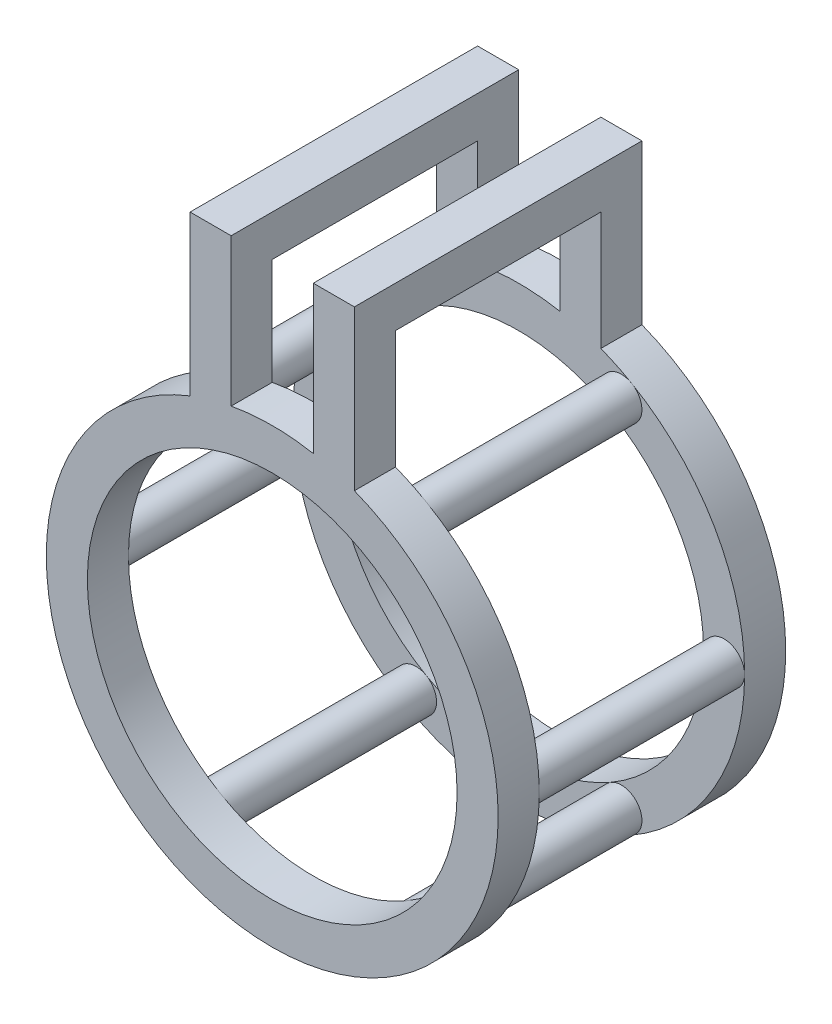
ISO-10303-21;
HEADER;
FILE_DESCRIPTION(('STEP AP214'),'2;1');
FILE_NAME('part.step','',(''),(''),'','','');
FILE_SCHEMA(('AUTOMOTIVE_DESIGN { 1 0 10303 214 1 1 1 1 }'));
ENDSEC;
DATA;
#1=APPLICATION_CONTEXT('core data for automotive mechanical design processes');
#2=APPLICATION_PROTOCOL_DEFINITION('international standard','automotive_design',2000,#1);
#3=PRODUCT_CONTEXT('',#1,'mechanical');
#4=PRODUCT('Part','Part','',(#3));
#5=PRODUCT_RELATED_PRODUCT_CATEGORY('part','',(#4));
#6=PRODUCT_DEFINITION_FORMATION('','',#4);
#7=PRODUCT_DEFINITION_CONTEXT('part definition',#1,'design');
#8=PRODUCT_DEFINITION('design','',#6,#7);
#9=PRODUCT_DEFINITION_SHAPE('','',#8);
#10=(LENGTH_UNIT() NAMED_UNIT(*) SI_UNIT(.MILLI.,.METRE.));
#11=(NAMED_UNIT(*) PLANE_ANGLE_UNIT() SI_UNIT($,.RADIAN.));
#12=(NAMED_UNIT(*) SI_UNIT($,.STERADIAN.) SOLID_ANGLE_UNIT());
#13=UNCERTAINTY_MEASURE_WITH_UNIT(LENGTH_MEASURE(1.E-05),#10,'distance_accuracy_value','');
#14=(GEOMETRIC_REPRESENTATION_CONTEXT(3) GLOBAL_UNCERTAINTY_ASSIGNED_CONTEXT((#13)) GLOBAL_UNIT_ASSIGNED_CONTEXT((#10,
#11,#12)) REPRESENTATION_CONTEXT('',''));
#15=CARTESIAN_POINT('',(0.,0.,0.));
#16=DIRECTION('',(0.,0.,1.));
#17=DIRECTION('',(1.,0.,0.));
#18=AXIS2_PLACEMENT_3D('',#15,#16,#17);
#19=CARTESIAN_POINT('',(0.,0.,-10.));
#20=DIRECTION('',(0.,0.,1.));
#21=DIRECTION('',(1.,0.,0.));
#22=AXIS2_PLACEMENT_3D('',#19,#20,#21);
#23=PLANE('',#22);
#24=CARTESIAN_POINT('',(-25.0000000000005,43.3012701892216,-10.));
#25=DIRECTION('',(0.,0.,-1.));
#26=DIRECTION('',(-1.,0.,0.));
#27=AXIS2_PLACEMENT_3D('',#24,#25,#26);
#28=CIRCLE('',#27,5.);
#29=CARTESIAN_POINT('',(-22.5000000000005,38.9711431702995,-10.));
#30=VERTEX_POINT('',#29);
#31=CARTESIAN_POINT('',(-27.5000000000006,47.6313972081438,-10.));
#32=VERTEX_POINT('',#31);
#33=EDGE_CURVE('E533',#30,#32,#28,.T.);
#34=ORIENTED_EDGE('',*,*,#33,.F.);
#35=CARTESIAN_POINT('',(0.,0.,-10.));
#36=DIRECTION('',(0.,0.,1.));
#37=DIRECTION('',(1.,0.,0.));
#38=AXIS2_PLACEMENT_3D('',#35,#36,#37);
#39=CIRCLE('',#38,45.);
#40=CARTESIAN_POINT('',(-45.,0.,-10.));
#41=VERTEX_POINT('',#40);
#42=EDGE_CURVE('E346',#30,#41,#39,.T.);
#43=ORIENTED_EDGE('',*,*,#42,.T.);
#44=CARTESIAN_POINT('',(-50.,0.,-10.));
#45=DIRECTION('',(0.,0.,-1.));
#46=DIRECTION('',(-1.,0.,0.));
#47=AXIS2_PLACEMENT_3D('',#44,#45,#46);
#48=CIRCLE('',#47,5.);
#49=CARTESIAN_POINT('',(-55.,0.,-10.));
#50=VERTEX_POINT('',#49);
#51=EDGE_CURVE('E505',#50,#41,#48,.T.);
#52=ORIENTED_EDGE('',*,*,#51,.F.);
#53=CARTESIAN_POINT('',(0.,0.,-10.));
#54=DIRECTION('',(0.,0.,1.));
#55=DIRECTION('',(1.,0.,0.));
#56=AXIS2_PLACEMENT_3D('',#53,#54,#55);
#57=CIRCLE('',#56,55.);
#58=EDGE_CURVE('E360',#32,#50,#57,.T.);
#59=ORIENTED_EDGE('',*,*,#58,.F.);
#60=EDGE_LOOP('',(#34,#43,#52,#59));
#61=FACE_BOUND('',#60,.T.);
#62=ADVANCED_FACE('F44',(#61),#23,.F.);
#63=CARTESIAN_POINT('',(10.,80.,-60.));
#64=DIRECTION('',(0.,0.,1.));
#65=DIRECTION('',(1.,0.,0.));
#66=AXIS2_PLACEMENT_3D('',#63,#64,#65);
#67=PLANE('',#66);
#68=CARTESIAN_POINT('',(0.,0.,-60.));
#69=DIRECTION('',(0.,0.,1.));
#70=DIRECTION('',(1.,0.,0.));
#71=AXIS2_PLACEMENT_3D('',#68,#69,#70);
#72=CIRCLE('',#71,45.);
#73=CARTESIAN_POINT('',(-22.5000000000005,38.9711431702995,-60.));
#74=VERTEX_POINT('',#73);
#75=CARTESIAN_POINT('',(-45.,0.,-60.));
#76=VERTEX_POINT('',#75);
#77=EDGE_CURVE('E245',#74,#76,#72,.T.);
#78=ORIENTED_EDGE('',*,*,#77,.F.);
#79=CARTESIAN_POINT('',(-25.0000000000005,43.3012701892216,-60.));
#80=DIRECTION('',(0.,0.,-1.));
#81=DIRECTION('',(-1.,0.,0.));
#82=AXIS2_PLACEMENT_3D('',#79,#80,#81);
#83=CIRCLE('',#82,5.);
#84=CARTESIAN_POINT('',(-27.5000000000006,47.6313972081438,-60.));
#85=VERTEX_POINT('',#84);
#86=EDGE_CURVE('E70',#74,#85,#83,.T.);
#87=ORIENTED_EDGE('',*,*,#86,.T.);
#88=CARTESIAN_POINT('',(0.,0.,-60.));
#89=DIRECTION('',(0.,0.,1.));
#90=DIRECTION('',(1.,0.,0.));
#91=AXIS2_PLACEMENT_3D('',#88,#89,#90);
#92=CIRCLE('',#91,55.);
#93=CARTESIAN_POINT('',(-55.,0.,-60.));
#94=VERTEX_POINT('',#93);
#95=EDGE_CURVE('E238',#85,#94,#92,.T.);
#96=ORIENTED_EDGE('',*,*,#95,.T.);
#97=CARTESIAN_POINT('',(-50.,0.,-60.));
#98=DIRECTION('',(0.,0.,-1.));
#99=DIRECTION('',(-1.,0.,0.));
#100=AXIS2_PLACEMENT_3D('',#97,#98,#99);
#101=CIRCLE('',#100,5.);
#102=EDGE_CURVE('E430',#94,#76,#101,.T.);
#103=ORIENTED_EDGE('',*,*,#102,.T.);
#104=EDGE_LOOP('',(#78,#87,#96,#103));
#105=FACE_BOUND('',#104,.T.);
#106=ADVANCED_FACE('F236',(#105),#67,.T.);
#107=EDGE_CURVE('E58',#32,#30,#28,.T.);
#108=ORIENTED_EDGE('',*,*,#107,.F.);
#109=CARTESIAN_POINT('',(-20.,51.234753829798,-10.));
#110=VERTEX_POINT('',#109);
#111=EDGE_CURVE('E358',#110,#32,#57,.T.);
#112=ORIENTED_EDGE('',*,*,#111,.F.);
#113=DIRECTION('',(0.,1.,0.));
#114=VECTOR('',#113,1.);
#115=CARTESIAN_POINT('',(-20.,51.234753829798,-10.));
#116=LINE('',#115,#114);
#117=CARTESIAN_POINT('',(-20.,80.,-10.));
#118=VERTEX_POINT('',#117);
#119=EDGE_CURVE('E421',#110,#118,#116,.T.);
#120=ORIENTED_EDGE('',*,*,#119,.T.);
#121=DIRECTION('',(-1.,0.,0.));
#122=VECTOR('',#121,1.);
#123=CARTESIAN_POINT('',(-10.,80.,-10.));
#124=LINE('',#123,#122);
#125=CARTESIAN_POINT('',(-10.,80.,-10.));
#126=VERTEX_POINT('',#125);
#127=EDGE_CURVE('E444',#126,#118,#124,.T.);
#128=ORIENTED_EDGE('',*,*,#127,.F.);
#129=DIRECTION('',(0.,1.,0.));
#130=VECTOR('',#129,1.);
#131=CARTESIAN_POINT('',(-10.,51.234753829798,-10.));
#132=LINE('',#131,#130);
#133=CARTESIAN_POINT('',(-10.,54.0832691319598,-10.));
#134=VERTEX_POINT('',#133);
#135=EDGE_CURVE('E437',#134,#126,#132,.T.);
#136=ORIENTED_EDGE('',*,*,#135,.F.);
#137=CARTESIAN_POINT('',(10.,54.0832691319598,-10.));
#138=VERTEX_POINT('',#137);
#139=EDGE_CURVE('E353',#138,#134,#57,.T.);
#140=ORIENTED_EDGE('',*,*,#139,.F.);
#141=DIRECTION('',(0.,1.,0.));
#142=VECTOR('',#141,1.);
#143=CARTESIAN_POINT('',(10.,45.,-10.));
#144=LINE('',#143,#142);
#145=CARTESIAN_POINT('',(10.,80.,-10.));
#146=VERTEX_POINT('',#145);
#147=EDGE_CURVE('E299',#138,#146,#144,.T.);
#148=ORIENTED_EDGE('',*,*,#147,.T.);
#149=DIRECTION('',(1.,0.,0.));
#150=VECTOR('',#149,1.);
#151=CARTESIAN_POINT('',(10.,80.,-10.));
#152=LINE('',#151,#150);
#153=CARTESIAN_POINT('',(20.,80.,-10.));
#154=VERTEX_POINT('',#153);
#155=EDGE_CURVE('E320',#146,#154,#152,.T.);
#156=ORIENTED_EDGE('',*,*,#155,.T.);
#157=DIRECTION('',(0.,1.,0.));
#158=VECTOR('',#157,1.);
#159=CARTESIAN_POINT('',(20.,45.,-10.));
#160=LINE('',#159,#158);
#161=CARTESIAN_POINT('',(20.,51.234753829798,-10.));
#162=VERTEX_POINT('',#161);
#163=EDGE_CURVE('E298',#162,#154,#160,.T.);
#164=ORIENTED_EDGE('',*,*,#163,.F.);
#165=CARTESIAN_POINT('',(27.4999999999996,47.6313972081444,-10.));
#166=VERTEX_POINT('',#165);
#167=EDGE_CURVE('E359',#166,#162,#57,.T.);
#168=ORIENTED_EDGE('',*,*,#167,.F.);
#169=CARTESIAN_POINT('',(24.9999999999996,43.3012701892222,-10.));
#170=DIRECTION('',(0.,0.,-1.));
#171=DIRECTION('',(-1.,0.,0.));
#172=AXIS2_PLACEMENT_3D('',#169,#170,#171);
#173=CIRCLE('',#172,4.99999999999999);
#174=CARTESIAN_POINT('',(22.4999999999996,38.9711431703,-10.));
#175=VERTEX_POINT('',#174);
#176=EDGE_CURVE('E232',#175,#166,#173,.T.);
#177=ORIENTED_EDGE('',*,*,#176,.F.);
#178=EDGE_CURVE('E1116',#175,#30,#39,.T.);
#179=ORIENTED_EDGE('',*,*,#178,.T.);
#180=EDGE_LOOP('',(#108,#112,#120,#128,#136,#140,#148,#156,#164,#168,#177,#179));
#181=FACE_BOUND('',#180,.T.);
#182=ADVANCED_FACE('F388',(#181),#23,.F.);
#183=CARTESIAN_POINT('',(-20.,51.234753829798,-60.));
#184=VERTEX_POINT('',#183);
#185=EDGE_CURVE('E247',#184,#85,#92,.T.);
#186=ORIENTED_EDGE('',*,*,#185,.T.);
#187=EDGE_CURVE('E230',#85,#74,#83,.T.);
#188=ORIENTED_EDGE('',*,*,#187,.T.);
#189=CARTESIAN_POINT('',(22.4999999999996,38.9711431703,-60.));
#190=VERTEX_POINT('',#189);
#191=EDGE_CURVE('E457',#190,#74,#72,.T.);
#192=ORIENTED_EDGE('',*,*,#191,.F.);
#193=CARTESIAN_POINT('',(24.9999999999996,43.3012701892222,-60.));
#194=DIRECTION('',(0.,0.,-1.));
#195=DIRECTION('',(-1.,0.,0.));
#196=AXIS2_PLACEMENT_3D('',#193,#194,#195);
#197=CIRCLE('',#196,4.99999999999999);
#198=CARTESIAN_POINT('',(27.4999999999996,47.6313972081444,-60.));
#199=VERTEX_POINT('',#198);
#200=EDGE_CURVE('E480',#190,#199,#197,.T.);
#201=ORIENTED_EDGE('',*,*,#200,.T.);
#202=CARTESIAN_POINT('',(20.,51.234753829798,-60.));
#203=VERTEX_POINT('',#202);
#204=EDGE_CURVE('E255',#199,#203,#92,.T.);
#205=ORIENTED_EDGE('',*,*,#204,.T.);
#206=DIRECTION('',(0.,-1.,0.));
#207=VECTOR('',#206,1.);
#208=CARTESIAN_POINT('',(20.,80.,-60.));
#209=LINE('',#208,#207);
#210=CARTESIAN_POINT('',(20.,80.,-60.));
#211=VERTEX_POINT('',#210);
#212=EDGE_CURVE('E325',#211,#203,#209,.T.);
#213=ORIENTED_EDGE('',*,*,#212,.F.);
#214=DIRECTION('',(1.,0.,0.));
#215=VECTOR('',#214,1.);
#216=CARTESIAN_POINT('',(10.,80.,-60.));
#217=LINE('',#216,#215);
#218=CARTESIAN_POINT('',(10.,80.,-60.));
#219=VERTEX_POINT('',#218);
#220=EDGE_CURVE('E340',#219,#211,#217,.T.);
#221=ORIENTED_EDGE('',*,*,#220,.F.);
#222=DIRECTION('',(0.,-1.,0.));
#223=VECTOR('',#222,1.);
#224=CARTESIAN_POINT('',(10.,80.,-60.));
#225=LINE('',#224,#223);
#226=CARTESIAN_POINT('',(10.,54.0832691319598,-60.));
#227=VERTEX_POINT('',#226);
#228=EDGE_CURVE('E308',#219,#227,#225,.T.);
#229=ORIENTED_EDGE('',*,*,#228,.T.);
#230=CARTESIAN_POINT('',(-10.,54.0832691319598,-60.));
#231=VERTEX_POINT('',#230);
#232=EDGE_CURVE('E254',#227,#231,#92,.T.);
#233=ORIENTED_EDGE('',*,*,#232,.T.);
#234=DIRECTION('',(0.,-1.,0.));
#235=VECTOR('',#234,1.);
#236=CARTESIAN_POINT('',(-10.,80.,-60.));
#237=LINE('',#236,#235);
#238=CARTESIAN_POINT('',(-10.,80.,-60.));
#239=VERTEX_POINT('',#238);
#240=EDGE_CURVE('E415',#239,#231,#237,.T.);
#241=ORIENTED_EDGE('',*,*,#240,.F.);
#242=DIRECTION('',(-1.,0.,0.));
#243=VECTOR('',#242,1.);
#244=CARTESIAN_POINT('',(-10.,80.,-60.));
#245=LINE('',#244,#243);
#246=CARTESIAN_POINT('',(-20.,80.,-60.));
#247=VERTEX_POINT('',#246);
#248=EDGE_CURVE('E442',#239,#247,#245,.T.);
#249=ORIENTED_EDGE('',*,*,#248,.T.);
#250=DIRECTION('',(0.,-1.,0.));
#251=VECTOR('',#250,1.);
#252=CARTESIAN_POINT('',(-20.,80.,-60.));
#253=LINE('',#252,#251);
#254=EDGE_CURVE('E259',#247,#184,#253,.T.);
#255=ORIENTED_EDGE('',*,*,#254,.T.);
#256=EDGE_LOOP('',(#186,#188,#192,#201,#205,#213,#221,#229,#233,#241,#249,#255));
#257=FACE_BOUND('',#256,.T.);
#258=ADVANCED_FACE('F258',(#257),#67,.T.);
#259=CARTESIAN_POINT('',(50.,3.49148133884313E-13,-10.));
#260=DIRECTION('',(0.,0.,-1.));
#261=DIRECTION('',(-1.,0.,0.));
#262=AXIS2_PLACEMENT_3D('',#259,#260,#261);
#263=CIRCLE('',#262,4.99999999999999);
#264=CARTESIAN_POINT('',(55.,3.84062947272745E-13,-10.));
#265=VERTEX_POINT('',#264);
#266=CARTESIAN_POINT('',(45.,3.14233320495882E-13,-10.));
#267=VERTEX_POINT('',#266);
#268=EDGE_CURVE('E478',#265,#267,#263,.T.);
#269=ORIENTED_EDGE('',*,*,#268,.F.);
#270=CARTESIAN_POINT('',(27.5000000000002,-47.631397208144,-10.));
#271=VERTEX_POINT('',#270);
#272=EDGE_CURVE('E538',#271,#265,#57,.T.);
#273=ORIENTED_EDGE('',*,*,#272,.F.);
#274=CARTESIAN_POINT('',(25.0000000000002,-43.3012701892218,-10.));
#275=DIRECTION('',(0.,0.,-1.));
#276=DIRECTION('',(-1.,0.,0.));
#277=AXIS2_PLACEMENT_3D('',#274,#275,#276);
#278=CIRCLE('',#277,5.);
#279=CARTESIAN_POINT('',(22.5000000000002,-38.9711431702996,-10.));
#280=VERTEX_POINT('',#279);
#281=EDGE_CURVE('E489',#280,#271,#278,.T.);
#282=ORIENTED_EDGE('',*,*,#281,.F.);
#283=EDGE_CURVE('E1120',#280,#267,#39,.T.);
#284=ORIENTED_EDGE('',*,*,#283,.T.);
#285=EDGE_LOOP('',(#269,#273,#282,#284));
#286=FACE_BOUND('',#285,.T.);
#287=ADVANCED_FACE('F547',(#286),#23,.F.);
#288=CARTESIAN_POINT('',(27.5000000000002,-47.631397208144,-60.));
#289=VERTEX_POINT('',#288);
#290=CARTESIAN_POINT('',(55.,3.84062947272745E-13,-60.));
#291=VERTEX_POINT('',#290);
#292=EDGE_CURVE('E269',#289,#291,#92,.T.);
#293=ORIENTED_EDGE('',*,*,#292,.T.);
#294=CARTESIAN_POINT('',(50.,3.49148133884313E-13,-60.));
#295=DIRECTION('',(0.,0.,-1.));
#296=DIRECTION('',(-1.,0.,0.));
#297=AXIS2_PLACEMENT_3D('',#294,#295,#296);
#298=CIRCLE('',#297,4.99999999999999);
#299=CARTESIAN_POINT('',(45.,3.14233320495882E-13,-60.));
#300=VERTEX_POINT('',#299);
#301=EDGE_CURVE('E466',#291,#300,#298,.T.);
#302=ORIENTED_EDGE('',*,*,#301,.T.);
#303=CARTESIAN_POINT('',(22.5000000000002,-38.9711431702996,-60.));
#304=VERTEX_POINT('',#303);
#305=EDGE_CURVE('E454',#304,#300,#72,.T.);
#306=ORIENTED_EDGE('',*,*,#305,.F.);
#307=CARTESIAN_POINT('',(25.0000000000002,-43.3012701892218,-60.));
#308=DIRECTION('',(0.,0.,-1.));
#309=DIRECTION('',(-1.,0.,0.));
#310=AXIS2_PLACEMENT_3D('',#307,#308,#309);
#311=CIRCLE('',#310,5.);
#312=EDGE_CURVE('E470',#304,#289,#311,.T.);
#313=ORIENTED_EDGE('',*,*,#312,.T.);
#314=EDGE_LOOP('',(#293,#302,#306,#313));
#315=FACE_BOUND('',#314,.T.);
#316=ADVANCED_FACE('F468',(#315),#67,.T.);
#317=EDGE_CURVE('E482',#271,#280,#278,.T.);
#318=ORIENTED_EDGE('',*,*,#317,.F.);
#319=CARTESIAN_POINT('',(-27.4999999999999,-47.6313972081442,-10.));
#320=VERTEX_POINT('',#319);
#321=EDGE_CURVE('E536',#320,#271,#57,.T.);
#322=ORIENTED_EDGE('',*,*,#321,.F.);
#323=CARTESIAN_POINT('',(-24.9999999999999,-43.301270189222,-10.));
#324=DIRECTION('',(0.,0.,-1.));
#325=DIRECTION('',(-1.,0.,0.));
#326=AXIS2_PLACEMENT_3D('',#323,#324,#325);
#327=CIRCLE('',#326,5.);
#328=CARTESIAN_POINT('',(-22.4999999999999,-38.9711431702998,-10.));
#329=VERTEX_POINT('',#328);
#330=EDGE_CURVE('E500',#329,#320,#327,.T.);
#331=ORIENTED_EDGE('',*,*,#330,.F.);
#332=EDGE_CURVE('E352',#329,#280,#39,.T.);
#333=ORIENTED_EDGE('',*,*,#332,.T.);
#334=EDGE_LOOP('',(#318,#322,#331,#333));
#335=FACE_BOUND('',#334,.T.);
#336=ADVANCED_FACE('F551',(#335),#23,.F.);
#337=CARTESIAN_POINT('',(-27.4999999999999,-47.6313972081442,-60.));
#338=VERTEX_POINT('',#337);
#339=EDGE_CURVE('E264',#338,#289,#92,.T.);
#340=ORIENTED_EDGE('',*,*,#339,.T.);
#341=EDGE_CURVE('E487',#289,#304,#311,.T.);
#342=ORIENTED_EDGE('',*,*,#341,.T.);
#343=CARTESIAN_POINT('',(-22.4999999999999,-38.9711431702998,-60.));
#344=VERTEX_POINT('',#343);
#345=EDGE_CURVE('E453',#344,#304,#72,.T.);
#346=ORIENTED_EDGE('',*,*,#345,.F.);
#347=CARTESIAN_POINT('',(-24.9999999999999,-43.301270189222,-60.));
#348=DIRECTION('',(0.,0.,-1.));
#349=DIRECTION('',(-1.,0.,0.));
#350=AXIS2_PLACEMENT_3D('',#347,#348,#349);
#351=CIRCLE('',#350,5.);
#352=EDGE_CURVE('E492',#344,#338,#351,.T.);
#353=ORIENTED_EDGE('',*,*,#352,.T.);
#354=EDGE_LOOP('',(#340,#342,#346,#353));
#355=FACE_BOUND('',#354,.T.);
#356=ADVANCED_FACE('F591',(#355),#67,.T.);
#357=EDGE_CURVE('E488',#320,#329,#327,.T.);
#358=ORIENTED_EDGE('',*,*,#357,.F.);
#359=EDGE_CURVE('E530',#50,#320,#57,.T.);
#360=ORIENTED_EDGE('',*,*,#359,.F.);
#361=EDGE_CURVE('E494',#41,#50,#48,.T.);
#362=ORIENTED_EDGE('',*,*,#361,.F.);
#363=EDGE_CURVE('E349',#41,#329,#39,.T.);
#364=ORIENTED_EDGE('',*,*,#363,.T.);
#365=EDGE_LOOP('',(#358,#360,#362,#364));
#366=FACE_BOUND('',#365,.T.);
#367=ADVANCED_FACE('F581',(#366),#23,.F.);
#368=EDGE_CURVE('E252',#94,#338,#92,.T.);
#369=ORIENTED_EDGE('',*,*,#368,.T.);
#370=EDGE_CURVE('E497',#338,#344,#351,.T.);
#371=ORIENTED_EDGE('',*,*,#370,.T.);
#372=EDGE_CURVE('E296',#76,#344,#72,.T.);
#373=ORIENTED_EDGE('',*,*,#372,.F.);
#374=EDGE_CURVE('E501',#76,#94,#101,.T.);
#375=ORIENTED_EDGE('',*,*,#374,.T.);
#376=EDGE_LOOP('',(#369,#371,#373,#375));
#377=FACE_BOUND('',#376,.T.);
#378=ADVANCED_FACE('F587',(#377),#67,.T.);
#379=CARTESIAN_POINT('',(0.,0.,-10.));
#380=DIRECTION('',(0.,0.,1.));
#381=DIRECTION('',(1.,0.,0.));
#382=AXIS2_PLACEMENT_3D('',#379,#380,#381);
#383=CYLINDRICAL_SURFACE('',#382,55.);
#384=ORIENTED_EDGE('',*,*,#139,.T.);
#385=DIRECTION('',(0.,0.,1.));
#386=VECTOR('',#385,1.);
#387=CARTESIAN_POINT('',(-10.,54.0832691319598,-10.));
#388=LINE('',#387,#386);
#389=CARTESIAN_POINT('',(-10.,54.0832691319598,0.));
#390=VERTEX_POINT('',#389);
#391=EDGE_CURVE('E446',#134,#390,#388,.T.);
#392=ORIENTED_EDGE('',*,*,#391,.T.);
#393=CARTESIAN_POINT('',(0.,0.,0.));
#394=DIRECTION('',(0.,0.,1.));
#395=DIRECTION('',(1.,0.,0.));
#396=AXIS2_PLACEMENT_3D('',#393,#394,#395);
#397=CIRCLE('',#396,55.);
#398=CARTESIAN_POINT('',(10.,54.0832691319598,0.));
#399=VERTEX_POINT('',#398);
#400=EDGE_CURVE('E356',#399,#390,#397,.T.);
#401=ORIENTED_EDGE('',*,*,#400,.F.);
#402=DIRECTION('',(0.,0.,1.));
#403=VECTOR('',#402,1.);
#404=CARTESIAN_POINT('',(10.,54.0832691319598,-10.));
#405=LINE('',#404,#403);
#406=EDGE_CURVE('E341',#399,#138,#405,.F.);
#407=ORIENTED_EDGE('',*,*,#406,.T.);
#408=EDGE_LOOP('',(#384,#392,#401,#407));
#409=FACE_BOUND('',#408,.T.);
#410=ADVANCED_FACE('F524',(#409),#383,.T.);
#411=CARTESIAN_POINT('',(0.,0.,-60.));
#412=DIRECTION('',(0.,0.,-1.));
#413=DIRECTION('',(-1.,0.,0.));
#414=AXIS2_PLACEMENT_3D('',#411,#412,#413);
#415=CYLINDRICAL_SURFACE('',#414,55.);
#416=DIRECTION('',(0.,0.,-1.));
#417=VECTOR('',#416,1.);
#418=CARTESIAN_POINT('',(-10.,54.0832691319598,-60.));
#419=LINE('',#418,#417);
#420=CARTESIAN_POINT('',(-10.,54.0832691319598,-70.));
#421=VERTEX_POINT('',#420);
#422=EDGE_CURVE('E11',#231,#421,#419,.T.);
#423=ORIENTED_EDGE('',*,*,#422,.F.);
#424=ORIENTED_EDGE('',*,*,#232,.F.);
#425=DIRECTION('',(0.,0.,-1.));
#426=VECTOR('',#425,1.);
#427=CARTESIAN_POINT('',(10.,54.0832691319598,-60.));
#428=LINE('',#427,#426);
#429=CARTESIAN_POINT('',(10.,54.0832691319599,-70.));
#430=VERTEX_POINT('',#429);
#431=EDGE_CURVE('E265',#227,#430,#428,.T.);
#432=ORIENTED_EDGE('',*,*,#431,.T.);
#433=CARTESIAN_POINT('',(0.,0.,-70.));
#434=DIRECTION('',(0.,0.,1.));
#435=DIRECTION('',(1.,0.,0.));
#436=AXIS2_PLACEMENT_3D('',#433,#434,#435);
#437=CIRCLE('',#436,55.);
#438=EDGE_CURVE('E284',#430,#421,#437,.T.);
#439=ORIENTED_EDGE('',*,*,#438,.T.);
#440=EDGE_LOOP('',(#423,#424,#432,#439));
#441=FACE_BOUND('',#440,.T.);
#442=ADVANCED_FACE('F401',(#441),#415,.T.);
#443=CARTESIAN_POINT('',(10.,0.,0.));
#444=DIRECTION('',(1.,0.,0.));
#445=DIRECTION('',(0.,0.,-1.));
#446=AXIS2_PLACEMENT_3D('',#443,#444,#445);
#447=PLANE('',#446);
#448=ORIENTED_EDGE('',*,*,#431,.F.);
#449=ORIENTED_EDGE('',*,*,#228,.F.);
#450=DIRECTION('',(0.,0.,-1.));
#451=VECTOR('',#450,1.);
#452=CARTESIAN_POINT('',(10.,80.,-10.));
#453=LINE('',#452,#451);
#454=EDGE_CURVE('E305',#146,#219,#453,.T.);
#455=ORIENTED_EDGE('',*,*,#454,.F.);
#456=ORIENTED_EDGE('',*,*,#147,.F.);
#457=ORIENTED_EDGE('',*,*,#406,.F.);
#458=DIRECTION('',(0.,-1.,0.));
#459=VECTOR('',#458,1.);
#460=CARTESIAN_POINT('',(10.,45.,0.));
#461=LINE('',#460,#459);
#462=CARTESIAN_POINT('',(10.,90.,0.));
#463=VERTEX_POINT('',#462);
#464=EDGE_CURVE('E314',#463,#399,#461,.T.);
#465=ORIENTED_EDGE('',*,*,#464,.F.);
#466=DIRECTION('',(0.,0.,1.));
#467=VECTOR('',#466,1.);
#468=CARTESIAN_POINT('',(10.,90.,0.));
#469=LINE('',#468,#467);
#470=CARTESIAN_POINT('',(10.,90.,-70.));
#471=VERTEX_POINT('',#470);
#472=EDGE_CURVE('E313',#471,#463,#469,.T.);
#473=ORIENTED_EDGE('',*,*,#472,.F.);
#474=DIRECTION('',(0.,1.,0.));
#475=VECTOR('',#474,1.);
#476=CARTESIAN_POINT('',(10.,90.,-70.));
#477=LINE('',#476,#475);
#478=EDGE_CURVE('E310',#430,#471,#477,.T.);
#479=ORIENTED_EDGE('',*,*,#478,.F.);
#480=EDGE_LOOP('',(#448,#449,#455,#456,#457,#465,#473,#479));
#481=FACE_BOUND('',#480,.T.);
#482=ADVANCED_FACE('F405',(#481),#447,.F.);
#483=CARTESIAN_POINT('',(20.,0.,0.));
#484=DIRECTION('',(1.,0.,0.));
#485=DIRECTION('',(0.,0.,-1.));
#486=AXIS2_PLACEMENT_3D('',#483,#484,#485);
#487=PLANE('',#486);
#488=ORIENTED_EDGE('',*,*,#212,.T.);
#489=DIRECTION('',(0.,0.,-1.));
#490=VECTOR('',#489,1.);
#491=CARTESIAN_POINT('',(20.,51.234753829798,-60.));
#492=LINE('',#491,#490);
#493=CARTESIAN_POINT('',(20.,51.234753829798,-70.));
#494=VERTEX_POINT('',#493);
#495=EDGE_CURVE('E52',#203,#494,#492,.T.);
#496=ORIENTED_EDGE('',*,*,#495,.T.);
#497=DIRECTION('',(0.,1.,0.));
#498=VECTOR('',#497,1.);
#499=CARTESIAN_POINT('',(20.,90.,-70.));
#500=LINE('',#499,#498);
#501=CARTESIAN_POINT('',(20.,90.,-70.));
#502=VERTEX_POINT('',#501);
#503=EDGE_CURVE('E322',#494,#502,#500,.T.);
#504=ORIENTED_EDGE('',*,*,#503,.T.);
#505=DIRECTION('',(0.,0.,1.));
#506=VECTOR('',#505,1.);
#507=CARTESIAN_POINT('',(20.,90.,0.));
#508=LINE('',#507,#506);
#509=CARTESIAN_POINT('',(20.,90.,0.));
#510=VERTEX_POINT('',#509);
#511=EDGE_CURVE('E326',#502,#510,#508,.T.);
#512=ORIENTED_EDGE('',*,*,#511,.T.);
#513=DIRECTION('',(0.,-1.,0.));
#514=VECTOR('',#513,1.);
#515=CARTESIAN_POINT('',(20.,45.,0.));
#516=LINE('',#515,#514);
#517=CARTESIAN_POINT('',(20.,51.234753829798,0.));
#518=VERTEX_POINT('',#517);
#519=EDGE_CURVE('E301',#510,#518,#516,.T.);
#520=ORIENTED_EDGE('',*,*,#519,.T.);
#521=DIRECTION('',(0.,0.,1.));
#522=VECTOR('',#521,1.);
#523=CARTESIAN_POINT('',(20.,51.234753829798,-10.));
#524=LINE('',#523,#522);
#525=EDGE_CURVE('E334',#518,#162,#524,.F.);
#526=ORIENTED_EDGE('',*,*,#525,.T.);
#527=ORIENTED_EDGE('',*,*,#163,.T.);
#528=DIRECTION('',(0.,0.,-1.));
#529=VECTOR('',#528,1.);
#530=CARTESIAN_POINT('',(20.,80.,-10.));
#531=LINE('',#530,#529);
#532=EDGE_CURVE('E317',#154,#211,#531,.T.);
#533=ORIENTED_EDGE('',*,*,#532,.T.);
#534=EDGE_LOOP('',(#488,#496,#504,#512,#520,#526,#527,#533));
#535=FACE_BOUND('',#534,.T.);
#536=ADVANCED_FACE('F365',(#535),#487,.T.);
#537=DIRECTION('',(0.,0.,-1.));
#538=VECTOR('',#537,1.);
#539=CARTESIAN_POINT('',(-20.,51.234753829798,0.));
#540=LINE('',#539,#538);
#541=CARTESIAN_POINT('',(-20.,51.234753829798,0.));
#542=VERTEX_POINT('',#541);
#543=EDGE_CURVE('E436',#542,#110,#540,.T.);
#544=ORIENTED_EDGE('',*,*,#543,.T.);
#545=ORIENTED_EDGE('',*,*,#111,.T.);
#546=ORIENTED_EDGE('',*,*,#58,.T.);
#547=ORIENTED_EDGE('',*,*,#359,.T.);
#548=ORIENTED_EDGE('',*,*,#321,.T.);
#549=ORIENTED_EDGE('',*,*,#272,.T.);
#550=EDGE_CURVE('E540',#265,#166,#57,.T.);
#551=ORIENTED_EDGE('',*,*,#550,.T.);
#552=ORIENTED_EDGE('',*,*,#167,.T.);
#553=ORIENTED_EDGE('',*,*,#525,.F.);
#554=EDGE_CURVE('E355',#542,#518,#397,.T.);
#555=ORIENTED_EDGE('',*,*,#554,.F.);
#556=EDGE_LOOP('',(#544,#545,#546,#547,#548,#549,#551,#552,#553,#555));
#557=FACE_BOUND('',#556,.T.);
#558=ADVANCED_FACE('F50',(#557),#383,.T.);
#559=EDGE_CURVE('E479',#166,#175,#173,.T.);
#560=ORIENTED_EDGE('',*,*,#559,.F.);
#561=ORIENTED_EDGE('',*,*,#550,.F.);
#562=EDGE_CURVE('E473',#267,#265,#263,.T.);
#563=ORIENTED_EDGE('',*,*,#562,.F.);
#564=EDGE_CURVE('E1117',#267,#175,#39,.T.);
#565=ORIENTED_EDGE('',*,*,#564,.T.);
#566=EDGE_LOOP('',(#560,#561,#563,#565));
#567=FACE_BOUND('',#566,.T.);
#568=ADVANCED_FACE('F573',(#567),#23,.F.);
#569=CARTESIAN_POINT('',(0.,0.,0.));
#570=DIRECTION('',(0.,0.,1.));
#571=DIRECTION('',(1.,0.,0.));
#572=AXIS2_PLACEMENT_3D('',#569,#570,#571);
#573=PLANE('',#572);
#574=ORIENTED_EDGE('',*,*,#400,.T.);
#575=DIRECTION('',(0.,-1.,0.));
#576=VECTOR('',#575,1.);
#577=CARTESIAN_POINT('',(-10.,90.,0.));
#578=LINE('',#577,#576);
#579=CARTESIAN_POINT('',(-10.,90.,0.));
#580=VERTEX_POINT('',#579);
#581=EDGE_CURVE('E412',#580,#390,#578,.T.);
#582=ORIENTED_EDGE('',*,*,#581,.F.);
#583=DIRECTION('',(-1.,0.,0.));
#584=VECTOR('',#583,1.);
#585=CARTESIAN_POINT('',(-10.,90.,0.));
#586=LINE('',#585,#584);
#587=CARTESIAN_POINT('',(-20.,90.,0.));
#588=VERTEX_POINT('',#587);
#589=EDGE_CURVE('E425',#580,#588,#586,.T.);
#590=ORIENTED_EDGE('',*,*,#589,.T.);
#591=DIRECTION('',(0.,-1.,0.));
#592=VECTOR('',#591,1.);
#593=CARTESIAN_POINT('',(-20.,90.,0.));
#594=LINE('',#593,#592);
#595=EDGE_CURVE('E383',#588,#542,#594,.T.);
#596=ORIENTED_EDGE('',*,*,#595,.T.);
#597=ORIENTED_EDGE('',*,*,#554,.T.);
#598=ORIENTED_EDGE('',*,*,#519,.F.);
#599=DIRECTION('',(1.,0.,0.));
#600=VECTOR('',#599,1.);
#601=CARTESIAN_POINT('',(10.,90.,0.));
#602=LINE('',#601,#600);
#603=EDGE_CURVE('E332',#463,#510,#602,.T.);
#604=ORIENTED_EDGE('',*,*,#603,.F.);
#605=ORIENTED_EDGE('',*,*,#464,.T.);
#606=EDGE_LOOP('',(#574,#582,#590,#596,#597,#598,#604,#605));
#607=FACE_BOUND('',#606,.T.);
#608=CARTESIAN_POINT('',(0.,0.,0.));
#609=DIRECTION('',(0.,0.,1.));
#610=DIRECTION('',(1.,0.,0.));
#611=AXIS2_PLACEMENT_3D('',#608,#609,#610);
#612=CIRCLE('',#611,45.);
#613=CARTESIAN_POINT('',(45.,0.,0.));
#614=VERTEX_POINT('',#613);
#615=EDGE_CURVE('E344',#614,#614,#612,.T.);
#616=ORIENTED_EDGE('',*,*,#615,.F.);
#617=EDGE_LOOP('',(#616));
#618=FACE_BOUND('',#617,.T.);
#619=ADVANCED_FACE('F378',(#607,#618),#573,.T.);
#620=CARTESIAN_POINT('',(0.,0.,-70.));
#621=DIRECTION('',(0.,0.,1.));
#622=DIRECTION('',(1.,0.,0.));
#623=AXIS2_PLACEMENT_3D('',#620,#621,#622);
#624=CYLINDRICAL_SURFACE('',#623,45.);
#625=ORIENTED_EDGE('',*,*,#615,.T.);
#626=EDGE_LOOP('',(#625));
#627=FACE_BOUND('',#626,.T.);
#628=ORIENTED_EDGE('',*,*,#363,.F.);
#629=ORIENTED_EDGE('',*,*,#42,.F.);
#630=ORIENTED_EDGE('',*,*,#178,.F.);
#631=ORIENTED_EDGE('',*,*,#564,.F.);
#632=ORIENTED_EDGE('',*,*,#283,.F.);
#633=ORIENTED_EDGE('',*,*,#332,.F.);
#634=EDGE_LOOP('',(#628,#629,#630,#631,#632,#633));
#635=FACE_BOUND('',#634,.T.);
#636=ADVANCED_FACE('F586',(#627,#635),#624,.F.);
#637=CARTESIAN_POINT('',(10.,90.,0.));
#638=DIRECTION('',(0.,1.,0.));
#639=DIRECTION('',(0.,0.,1.));
#640=AXIS2_PLACEMENT_3D('',#637,#638,#639);
#641=PLANE('',#640);
#642=ORIENTED_EDGE('',*,*,#511,.F.);
#643=DIRECTION('',(1.,0.,0.));
#644=VECTOR('',#643,1.);
#645=CARTESIAN_POINT('',(10.,90.,-70.));
#646=LINE('',#645,#644);
#647=EDGE_CURVE('E331',#471,#502,#646,.T.);
#648=ORIENTED_EDGE('',*,*,#647,.F.);
#649=ORIENTED_EDGE('',*,*,#472,.T.);
#650=ORIENTED_EDGE('',*,*,#603,.T.);
#651=EDGE_LOOP('',(#642,#648,#649,#650));
#652=FACE_BOUND('',#651,.T.);
#653=ADVANCED_FACE('F374',(#652),#641,.T.);
#654=CARTESIAN_POINT('',(10.,90.,-70.));
#655=DIRECTION('',(0.,0.,-1.));
#656=DIRECTION('',(-1.,0.,0.));
#657=AXIS2_PLACEMENT_3D('',#654,#655,#656);
#658=PLANE('',#657);
#659=CARTESIAN_POINT('',(-20.,51.234753829798,-70.));
#660=VERTEX_POINT('',#659);
#661=EDGE_CURVE('E292',#660,#494,#437,.T.);
#662=ORIENTED_EDGE('',*,*,#661,.F.);
#663=DIRECTION('',(0.,1.,0.));
#664=VECTOR('',#663,1.);
#665=CARTESIAN_POINT('',(-20.,51.234753829798,-70.));
#666=LINE('',#665,#664);
#667=CARTESIAN_POINT('',(-20.,90.,-70.));
#668=VERTEX_POINT('',#667);
#669=EDGE_CURVE('E431',#660,#668,#666,.T.);
#670=ORIENTED_EDGE('',*,*,#669,.T.);
#671=DIRECTION('',(-1.,0.,0.));
#672=VECTOR('',#671,1.);
#673=CARTESIAN_POINT('',(-10.,90.,-70.));
#674=LINE('',#673,#672);
#675=CARTESIAN_POINT('',(-10.,90.,-70.));
#676=VERTEX_POINT('',#675);
#677=EDGE_CURVE('E407',#676,#668,#674,.T.);
#678=ORIENTED_EDGE('',*,*,#677,.F.);
#679=DIRECTION('',(0.,1.,0.));
#680=VECTOR('',#679,1.);
#681=CARTESIAN_POINT('',(-10.,51.234753829798,-70.));
#682=LINE('',#681,#680);
#683=EDGE_CURVE('E406',#421,#676,#682,.T.);
#684=ORIENTED_EDGE('',*,*,#683,.F.);
#685=ORIENTED_EDGE('',*,*,#438,.F.);
#686=ORIENTED_EDGE('',*,*,#478,.T.);
#687=ORIENTED_EDGE('',*,*,#647,.T.);
#688=ORIENTED_EDGE('',*,*,#503,.F.);
#689=EDGE_LOOP('',(#662,#670,#678,#684,#685,#686,#687,#688));
#690=FACE_BOUND('',#689,.T.);
#691=CARTESIAN_POINT('',(0.,0.,-70.));
#692=DIRECTION('',(0.,0.,1.));
#693=DIRECTION('',(1.,0.,0.));
#694=AXIS2_PLACEMENT_3D('',#691,#692,#693);
#695=CIRCLE('',#694,45.);
#696=CARTESIAN_POINT('',(45.,0.,-70.));
#697=VERTEX_POINT('',#696);
#698=EDGE_CURVE('E447',#697,#697,#695,.T.);
#699=ORIENTED_EDGE('',*,*,#698,.T.);
#700=EDGE_LOOP('',(#699));
#701=FACE_BOUND('',#700,.T.);
#702=ADVANCED_FACE('F369',(#690,#701),#658,.T.);
#703=EDGE_CURVE('E274',#291,#199,#92,.T.);
#704=ORIENTED_EDGE('',*,*,#703,.T.);
#705=EDGE_CURVE('E475',#199,#190,#197,.T.);
#706=ORIENTED_EDGE('',*,*,#705,.T.);
#707=EDGE_CURVE('E456',#300,#190,#72,.T.);
#708=ORIENTED_EDGE('',*,*,#707,.F.);
#709=EDGE_CURVE('E469',#300,#291,#298,.T.);
#710=ORIENTED_EDGE('',*,*,#709,.T.);
#711=EDGE_LOOP('',(#704,#706,#708,#710));
#712=FACE_BOUND('',#711,.T.);
#713=ADVANCED_FACE('F471',(#712),#67,.T.);
#714=CARTESIAN_POINT('',(10.,80.,-10.));
#715=DIRECTION('',(0.,-1.,0.));
#716=DIRECTION('',(0.,0.,-1.));
#717=AXIS2_PLACEMENT_3D('',#714,#715,#716);
#718=PLANE('',#717);
#719=ORIENTED_EDGE('',*,*,#532,.F.);
#720=ORIENTED_EDGE('',*,*,#155,.F.);
#721=ORIENTED_EDGE('',*,*,#454,.T.);
#722=ORIENTED_EDGE('',*,*,#220,.T.);
#723=EDGE_LOOP('',(#719,#720,#721,#722));
#724=FACE_BOUND('',#723,.T.);
#725=ADVANCED_FACE('F396',(#724),#718,.T.);
#726=ORIENTED_EDGE('',*,*,#185,.F.);
#727=DIRECTION('',(0.,0.,-1.));
#728=VECTOR('',#727,1.);
#729=CARTESIAN_POINT('',(-20.,51.234753829798,-60.));
#730=LINE('',#729,#728);
#731=EDGE_CURVE('E370',#184,#660,#730,.T.);
#732=ORIENTED_EDGE('',*,*,#731,.T.);
#733=ORIENTED_EDGE('',*,*,#661,.T.);
#734=ORIENTED_EDGE('',*,*,#495,.F.);
#735=ORIENTED_EDGE('',*,*,#204,.F.);
#736=ORIENTED_EDGE('',*,*,#703,.F.);
#737=ORIENTED_EDGE('',*,*,#292,.F.);
#738=ORIENTED_EDGE('',*,*,#339,.F.);
#739=ORIENTED_EDGE('',*,*,#368,.F.);
#740=ORIENTED_EDGE('',*,*,#95,.F.);
#741=EDGE_LOOP('',(#726,#732,#733,#734,#735,#736,#737,#738,#739,#740));
#742=FACE_BOUND('',#741,.T.);
#743=ADVANCED_FACE('F250',(#742),#415,.T.);
#744=CARTESIAN_POINT('',(0.,0.,-70.));
#745=DIRECTION('',(0.,0.,1.));
#746=DIRECTION('',(1.,0.,0.));
#747=AXIS2_PLACEMENT_3D('',#744,#745,#746);
#748=CYLINDRICAL_SURFACE('',#747,45.);
#749=ORIENTED_EDGE('',*,*,#372,.T.);
#750=ORIENTED_EDGE('',*,*,#345,.T.);
#751=ORIENTED_EDGE('',*,*,#305,.T.);
#752=ORIENTED_EDGE('',*,*,#707,.T.);
#753=ORIENTED_EDGE('',*,*,#191,.T.);
#754=ORIENTED_EDGE('',*,*,#77,.T.);
#755=EDGE_LOOP('',(#749,#750,#751,#752,#753,#754));
#756=FACE_BOUND('',#755,.T.);
#757=ORIENTED_EDGE('',*,*,#698,.F.);
#758=EDGE_LOOP('',(#757));
#759=FACE_BOUND('',#758,.T.);
#760=ADVANCED_FACE('F462',(#756,#759),#748,.F.);
#761=CARTESIAN_POINT('',(-10.,0.,0.));
#762=DIRECTION('',(-1.,0.,0.));
#763=DIRECTION('',(0.,0.,1.));
#764=AXIS2_PLACEMENT_3D('',#761,#762,#763);
#765=PLANE('',#764);
#766=ORIENTED_EDGE('',*,*,#391,.F.);
#767=ORIENTED_EDGE('',*,*,#135,.T.);
#768=DIRECTION('',(0.,0.,-1.));
#769=VECTOR('',#768,1.);
#770=CARTESIAN_POINT('',(-10.,80.,-10.));
#771=LINE('',#770,#769);
#772=EDGE_CURVE('E418',#126,#239,#771,.T.);
#773=ORIENTED_EDGE('',*,*,#772,.T.);
#774=ORIENTED_EDGE('',*,*,#240,.T.);
#775=ORIENTED_EDGE('',*,*,#422,.T.);
#776=ORIENTED_EDGE('',*,*,#683,.T.);
#777=DIRECTION('',(0.,0.,1.));
#778=VECTOR('',#777,1.);
#779=CARTESIAN_POINT('',(-10.,90.,-70.));
#780=LINE('',#779,#778);
#781=EDGE_CURVE('E413',#676,#580,#780,.T.);
#782=ORIENTED_EDGE('',*,*,#781,.T.);
#783=ORIENTED_EDGE('',*,*,#581,.T.);
#784=EDGE_LOOP('',(#766,#767,#773,#774,#775,#776,#782,#783));
#785=FACE_BOUND('',#784,.T.);
#786=ADVANCED_FACE('F506',(#785),#765,.F.);
#787=CARTESIAN_POINT('',(-10.,80.,-10.));
#788=DIRECTION('',(0.,1.,0.));
#789=DIRECTION('',(0.,0.,1.));
#790=AXIS2_PLACEMENT_3D('',#787,#788,#789);
#791=PLANE('',#790);
#792=DIRECTION('',(0.,0.,-1.));
#793=VECTOR('',#792,1.);
#794=CARTESIAN_POINT('',(-20.,80.,-10.));
#795=LINE('',#794,#793);
#796=EDGE_CURVE('E426',#118,#247,#795,.T.);
#797=ORIENTED_EDGE('',*,*,#796,.T.);
#798=ORIENTED_EDGE('',*,*,#248,.F.);
#799=ORIENTED_EDGE('',*,*,#772,.F.);
#800=ORIENTED_EDGE('',*,*,#127,.T.);
#801=EDGE_LOOP('',(#797,#798,#799,#800));
#802=FACE_BOUND('',#801,.T.);
#803=ADVANCED_FACE('F511',(#802),#791,.F.);
#804=CARTESIAN_POINT('',(-10.,90.,-70.));
#805=DIRECTION('',(0.,-1.,0.));
#806=DIRECTION('',(0.,0.,-1.));
#807=AXIS2_PLACEMENT_3D('',#804,#805,#806);
#808=PLANE('',#807);
#809=DIRECTION('',(0.,0.,1.));
#810=VECTOR('',#809,1.);
#811=CARTESIAN_POINT('',(-20.,90.,-70.));
#812=LINE('',#811,#810);
#813=EDGE_CURVE('E433',#668,#588,#812,.T.);
#814=ORIENTED_EDGE('',*,*,#813,.T.);
#815=ORIENTED_EDGE('',*,*,#589,.F.);
#816=ORIENTED_EDGE('',*,*,#781,.F.);
#817=ORIENTED_EDGE('',*,*,#677,.T.);
#818=EDGE_LOOP('',(#814,#815,#816,#817));
#819=FACE_BOUND('',#818,.T.);
#820=ADVANCED_FACE('F518',(#819),#808,.F.);
#821=CARTESIAN_POINT('',(-20.,0.,0.));
#822=DIRECTION('',(-1.,0.,0.));
#823=DIRECTION('',(0.,0.,1.));
#824=AXIS2_PLACEMENT_3D('',#821,#822,#823);
#825=PLANE('',#824);
#826=ORIENTED_EDGE('',*,*,#119,.F.);
#827=ORIENTED_EDGE('',*,*,#543,.F.);
#828=ORIENTED_EDGE('',*,*,#595,.F.);
#829=ORIENTED_EDGE('',*,*,#813,.F.);
#830=ORIENTED_EDGE('',*,*,#669,.F.);
#831=ORIENTED_EDGE('',*,*,#731,.F.);
#832=ORIENTED_EDGE('',*,*,#254,.F.);
#833=ORIENTED_EDGE('',*,*,#796,.F.);
#834=EDGE_LOOP('',(#826,#827,#828,#829,#830,#831,#832,#833));
#835=FACE_BOUND('',#834,.T.);
#836=ADVANCED_FACE('F516',(#835),#825,.T.);
#837=CARTESIAN_POINT('',(-50.,0.,-60.));
#838=DIRECTION('',(0.,0.,1.));
#839=DIRECTION('',(1.,0.,0.));
#840=AXIS2_PLACEMENT_3D('',#837,#838,#839);
#841=CYLINDRICAL_SURFACE('',#840,5.);
#842=ORIENTED_EDGE('',*,*,#102,.F.);
#843=ORIENTED_EDGE('',*,*,#374,.F.);
#844=EDGE_LOOP('',(#842,#843));
#845=FACE_BOUND('',#844,.T.);
#846=ORIENTED_EDGE('',*,*,#51,.T.);
#847=ORIENTED_EDGE('',*,*,#361,.T.);
#848=EDGE_LOOP('',(#846,#847));
#849=FACE_BOUND('',#848,.T.);
#850=ADVANCED_FACE('F569',(#845,#849),#841,.T.);
#851=CARTESIAN_POINT('',(-24.9999999999999,-43.301270189222,-60.));
#852=DIRECTION('',(0.,0.,1.));
#853=DIRECTION('',(1.,0.,0.));
#854=AXIS2_PLACEMENT_3D('',#851,#852,#853);
#855=CYLINDRICAL_SURFACE('',#854,5.);
#856=ORIENTED_EDGE('',*,*,#352,.F.);
#857=ORIENTED_EDGE('',*,*,#370,.F.);
#858=EDGE_LOOP('',(#856,#857));
#859=FACE_BOUND('',#858,.T.);
#860=ORIENTED_EDGE('',*,*,#330,.T.);
#861=ORIENTED_EDGE('',*,*,#357,.T.);
#862=EDGE_LOOP('',(#860,#861));
#863=FACE_BOUND('',#862,.T.);
#864=ADVANCED_FACE('F559',(#859,#863),#855,.T.);
#865=CARTESIAN_POINT('',(25.0000000000002,-43.3012701892218,-60.));
#866=DIRECTION('',(0.,0.,1.));
#867=DIRECTION('',(1.,0.,0.));
#868=AXIS2_PLACEMENT_3D('',#865,#866,#867);
#869=CYLINDRICAL_SURFACE('',#868,5.);
#870=ORIENTED_EDGE('',*,*,#312,.F.);
#871=ORIENTED_EDGE('',*,*,#341,.F.);
#872=EDGE_LOOP('',(#870,#871));
#873=FACE_BOUND('',#872,.T.);
#874=ORIENTED_EDGE('',*,*,#281,.T.);
#875=ORIENTED_EDGE('',*,*,#317,.T.);
#876=EDGE_LOOP('',(#874,#875));
#877=FACE_BOUND('',#876,.T.);
#878=ADVANCED_FACE('F560',(#873,#877),#869,.T.);
#879=CARTESIAN_POINT('',(50.,3.49148133884313E-13,-60.));
#880=DIRECTION('',(0.,0.,1.));
#881=DIRECTION('',(1.,0.,0.));
#882=AXIS2_PLACEMENT_3D('',#879,#880,#881);
#883=CYLINDRICAL_SURFACE('',#882,4.99999999999999);
#884=ORIENTED_EDGE('',*,*,#709,.F.);
#885=ORIENTED_EDGE('',*,*,#301,.F.);
#886=EDGE_LOOP('',(#884,#885));
#887=FACE_BOUND('',#886,.T.);
#888=ORIENTED_EDGE('',*,*,#562,.T.);
#889=ORIENTED_EDGE('',*,*,#268,.T.);
#890=EDGE_LOOP('',(#888,#889));
#891=FACE_BOUND('',#890,.T.);
#892=ADVANCED_FACE('F558',(#887,#891),#883,.T.);
#893=CARTESIAN_POINT('',(24.9999999999996,43.3012701892222,-60.));
#894=DIRECTION('',(0.,0.,1.));
#895=DIRECTION('',(1.,0.,0.));
#896=AXIS2_PLACEMENT_3D('',#893,#894,#895);
#897=CYLINDRICAL_SURFACE('',#896,4.99999999999999);
#898=ORIENTED_EDGE('',*,*,#705,.F.);
#899=ORIENTED_EDGE('',*,*,#200,.F.);
#900=EDGE_LOOP('',(#898,#899));
#901=FACE_BOUND('',#900,.T.);
#902=ORIENTED_EDGE('',*,*,#559,.T.);
#903=ORIENTED_EDGE('',*,*,#176,.T.);
#904=EDGE_LOOP('',(#902,#903));
#905=FACE_BOUND('',#904,.T.);
#906=ADVANCED_FACE('F570',(#901,#905),#897,.T.);
#907=CARTESIAN_POINT('',(-25.0000000000005,43.3012701892216,-60.));
#908=DIRECTION('',(0.,0.,1.));
#909=DIRECTION('',(1.,0.,0.));
#910=AXIS2_PLACEMENT_3D('',#907,#908,#909);
#911=CYLINDRICAL_SURFACE('',#910,5.);
#912=ORIENTED_EDGE('',*,*,#187,.F.);
#913=ORIENTED_EDGE('',*,*,#86,.F.);
#914=EDGE_LOOP('',(#912,#913));
#915=FACE_BOUND('',#914,.T.);
#916=ORIENTED_EDGE('',*,*,#107,.T.);
#917=ORIENTED_EDGE('',*,*,#33,.T.);
#918=EDGE_LOOP('',(#916,#917));
#919=FACE_BOUND('',#918,.T.);
#920=ADVANCED_FACE('F227',(#915,#919),#911,.T.);
#921=CLOSED_SHELL('',(#62,#106,#182,#258,#287,#316,#336,#356,#367,#378,#410,#442,#482,#536,#558,
#568,#619,#636,#653,#702,#713,#725,#743,#760,#786,#803,#820,#836,#850,#864,#878,#892,#906,#920));
#922=MANIFOLD_SOLID_BREP('B2',#921);
#923=ADVANCED_BREP_SHAPE_REPRESENTATION('',(#18,#922),#14);
#924=SHAPE_DEFINITION_REPRESENTATION(#9,#923);
ENDSEC;
END-ISO-10303-21;
